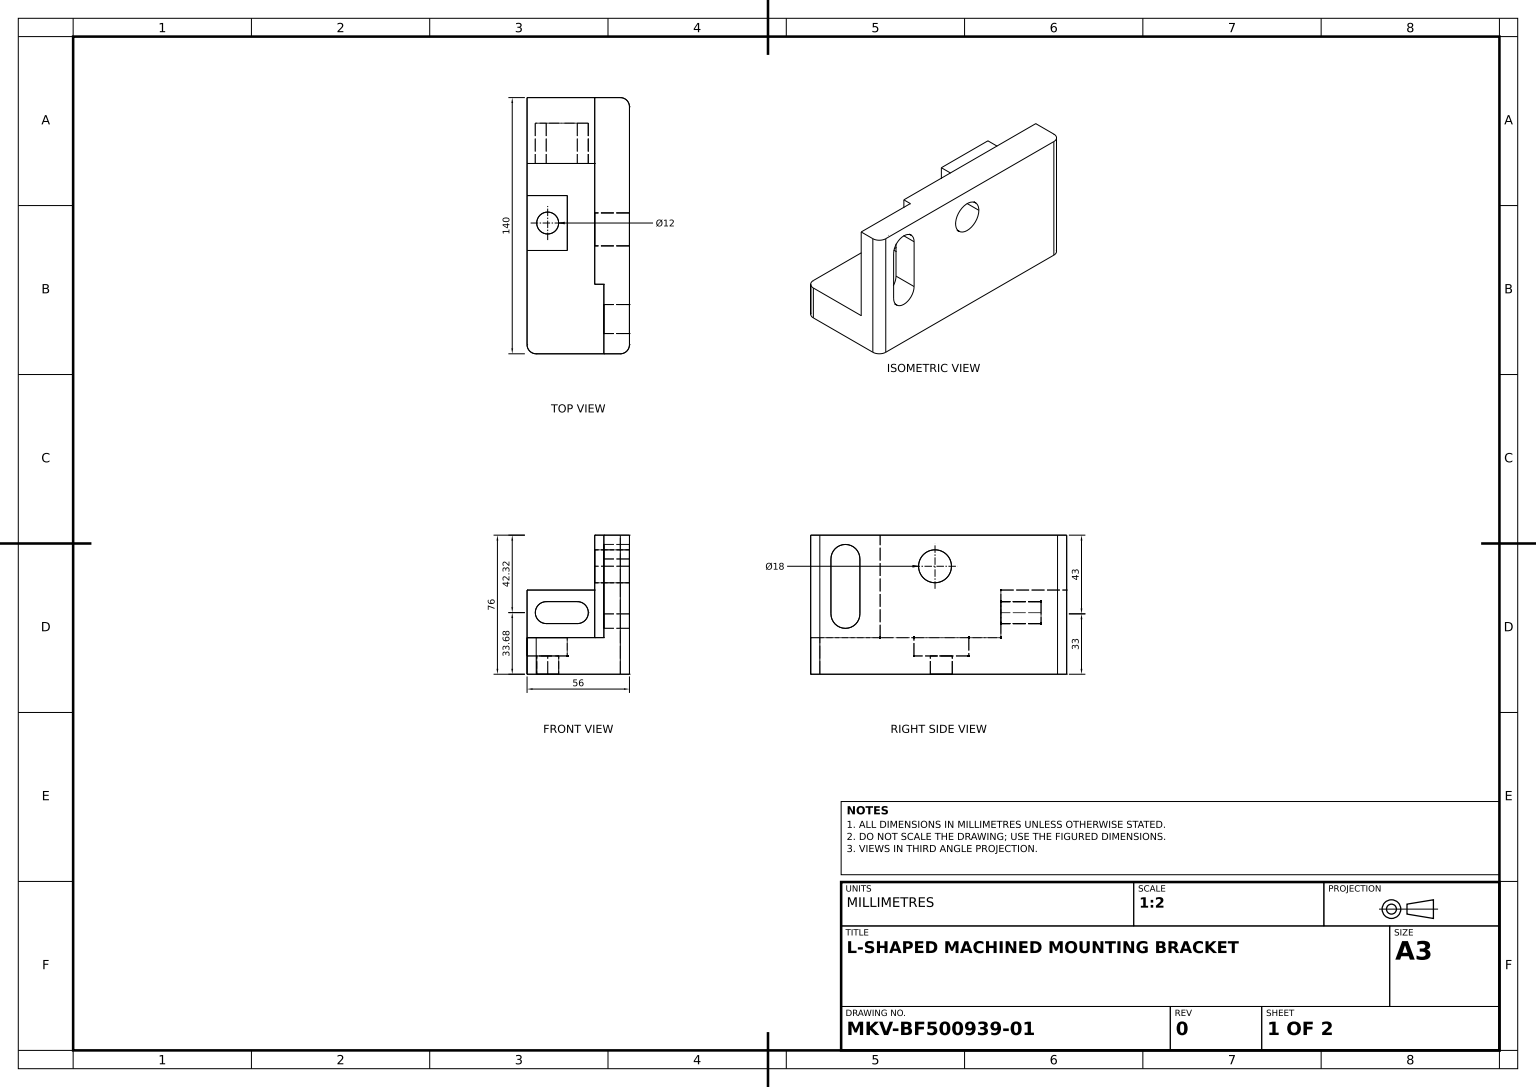
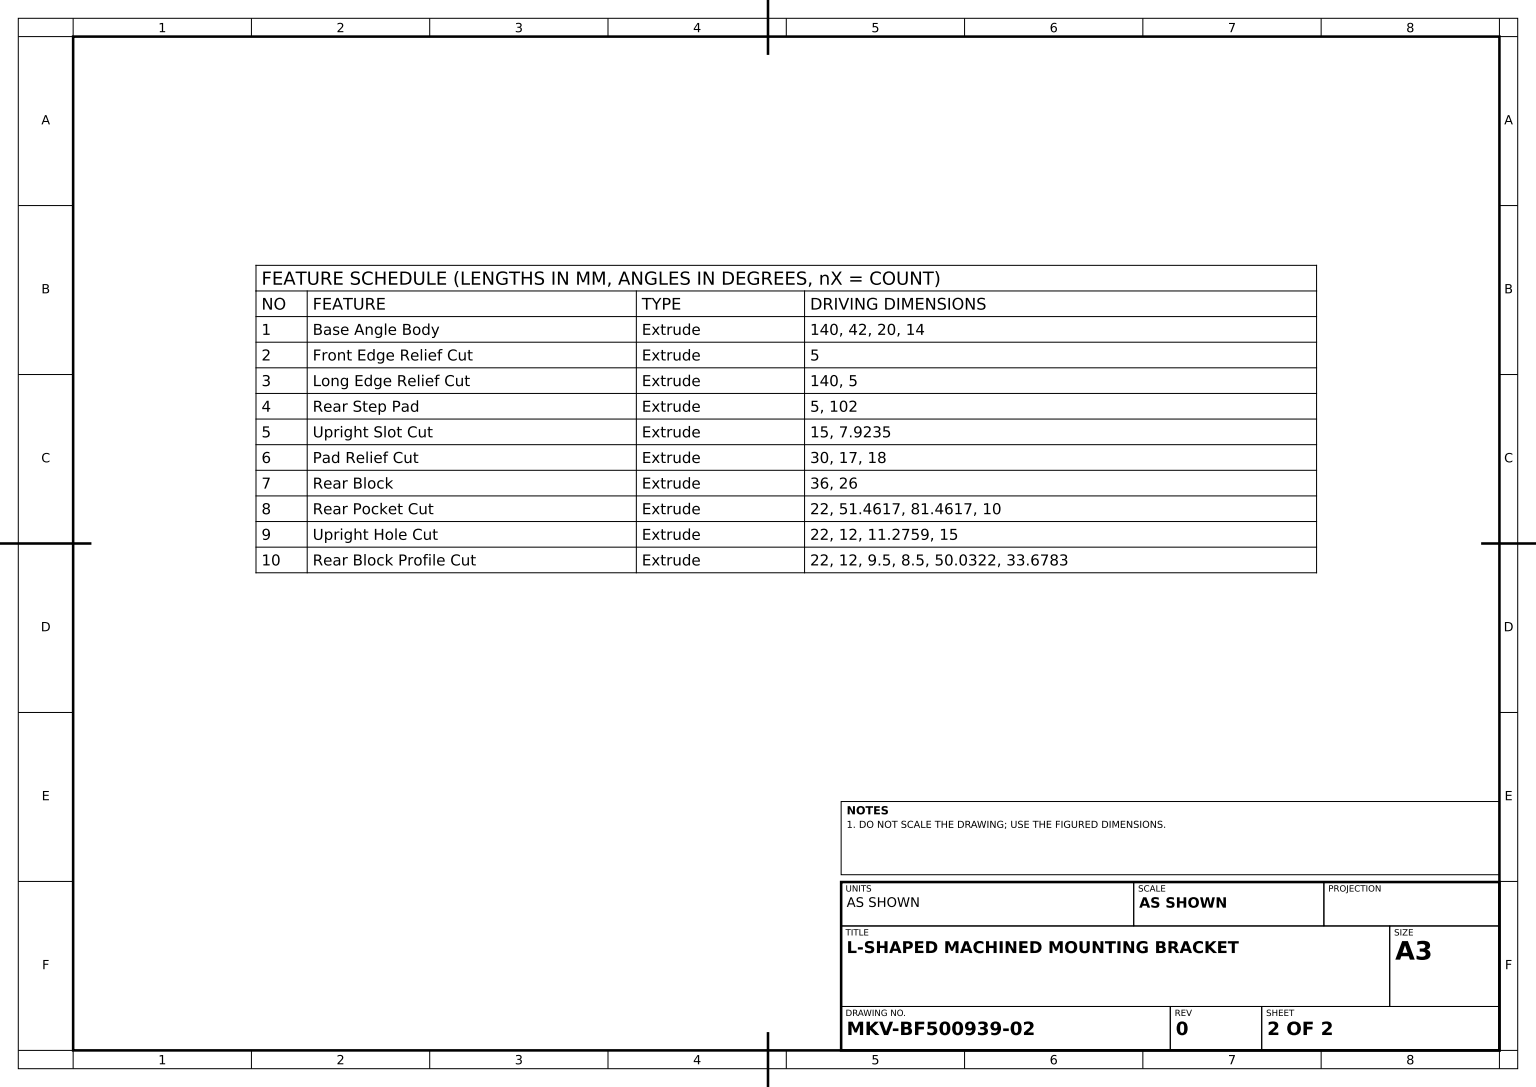
SolidWorks part; units mm, degrees
material "Plain Carbon Steel"
ref_plane "Front Plane" through (0, 0, 0) normal (0, 0, 1) x (1, 0, 0)
ref_plane "Top Plane" through (0, 0, 0) normal (0, 1, 0) x (1, 0, 0)
ref_plane "Right Plane" through (0, 0, 0) normal (1, 0, 0) x (0, 0, -1)
sketch "Base Angle Profile Sketch" plane through (0, 0, 0) normal (0, 0, 1) x (1, 0, 0)
  line L0 (0, 0) -> (-56, 0)
  line L1 (-56, 0) -> (-56, 20)
  line L2 (-56, 20) -> (-14, 20)
  line L3 (-14, 20) -> (-14, 76)
  line L4 (-14, 76) -> (0, 76)
  line L5 (0, 76) -> (0, 0)
  dimension "D1" = 42
  dimension "D2" = 20
  dimension "D3" = 14
extrude "Base Angle Body" add sketch "Base Angle Profile Sketch" along normal mid plane 140
sketch "Front Edge Relief Sketch" plane through (0, 76, 0) normal (0, 1, 0) x (1, 0, 0)
  line L0 (-5, 70) -> (0, 70)
  line L2 (0, 70) -> (0, 65)
  line L4 (0, 0) -> (-56, 0) construction
  line L5 (-56, -70) -> (-56, 70) construction
  line L6 (0, -70) -> (0, -65)
  line L7 (-5, -70) -> (0, -70)
  arc A0 (0, 65) -> (-5, 70) centre (-5, 65) ccw
  arc A1 (0, -65) -> (-5, -70) centre (-5, -65) cw
  dimension "D1" = 5
extrude "Front Edge Relief Cut" cut sketch "Front Edge Relief Sketch" against normal through all
sketch "Long Edge Relief Sketch" plane through (0, 20, 0) normal (0, 1, 0) x (1, 0, 0)
  line L0 (-56, -65) -> (-56, -70)
  line L2 (-56, -70) -> (-51, -70)
  arc A0 (-56, -65) -> (-51, -70) centre (-51, -65) ccw
  dimension "D1" = 5
extrude "Long Edge Relief Cut" cut sketch "Long Edge Relief Sketch" against normal blind 140
sketch "Rear Step Pad Sketch" plane through (-14, 0, 0) normal (-1, 0, 0) x (0, 0, 1)
  line L2 (70, 76) -> (-70, 76) construction
  line L3 (32, 76) -> (32, 20)
  line L4 (65, 20) -> (-70, 20) construction
  line L6 (32, 76) -> (-70, 76)
  line L7 (-70, 76) -> (-70, 20)
  line L8 (-70, 20) -> (32, 20)
  line L9 (-70, 76) -> (-70, 20) construction
  dimension "D1" = 102
extrude "Rear Step Pad" add sketch "Rear Step Pad Sketch" along normal blind 5
sketch "Upright Slot Sketch" plane through (-14, 0, 0) normal (-1, 0, 0) x (0, 0, 1)
  line L0 (51, 76) -> (51, 20) construction
  line L1 (70, 76) -> (32, 76) construction
  line L2 (70, 20) -> (32, 20) construction
  line L3 (51, 33) -> (51, 63) construction
  line L4 (43.0765, 33) -> (43.0765, 63)
  line L5 (58.9235, 33) -> (58.9235, 63)
  arc A0 (43.0765, 33) -> (58.9235, 33) centre (51, 33) ccw
  arc A1 (58.9235, 63) -> (43.0765, 63) centre (51, 63) ccw
  point P8 (51, 48)
  dimension "D2" = 7.9235
  dimension "D1" = 15
extrude "Upright Slot Cut" cut sketch "Upright Slot Sketch" against normal through all
sketch "Pad Relief Sketch" plane through (-19, 0, 0) normal (-1, 0, 0) x (0, 0, 1)
  line L0 (32, 76) -> (2, 76) construction
  line L1 (32, 76) -> (-70, 76) construction
  line L2 (2, 76) -> (2, 59) construction
  circle A0 centre (2, 59) radius 9
  dimension "D1" = 30
  dimension "D3" = 18
  dimension "D2" = 17
extrude "Pad Relief Cut" cut sketch "Pad Relief Sketch" against normal through all
sketch "Rear Block Sketch" plane through (0, 0, -70) normal (0, 0, -1) x (-1, 0, 0)
  line L0 (56, 20) -> (56, 46)
  line L1 (56, 46) -> (19, 46)
  line L2 (19, 76) -> (19, 20) construction
  line L3 (19, 46) -> (19, 20)
  line L4 (19, 20) -> (56, 20)
  line L5 (19, 20) -> (56, 20) construction
  dimension "D1" = 26
extrude "Rear Block" add sketch "Rear Block Sketch" against normal blind 36
sketch "Rear Pocket Sketch" plane through (-56, 0, 0) normal (-1, 0, 0) x (0, 0, 1)
  line L0 (65, 20) -> (-34, 20) construction
  line L1 (-34, 20) -> (32, 20) construction
  line L2 (-16.4617, 20) -> (-16.4617, 10)
  line L3 (-16.4617, 10) -> (13.5383, 10)
  line L4 (13.5383, 10) -> (13.5383, 20)
  line L5 (-16.4617, 20) -> (13.5383, 20)
  dimension "D1" = 51.4617
  dimension "D2" = 81.4617
  dimension "D3" = 10
extrude "Rear Pocket Cut" cut sketch "Rear Pocket Sketch" against normal blind 22
sketch "Upright Hole Sketch" plane through (0, 10, 0) normal (0, 1, 0) x (1, 0, 0)
  line L0 (-56, 16.4617) -> (-56, -13.5383) construction
  circle A0 centre (-44.7241, 1.4617) radius 6
  dimension "D1" = 12
  dimension "D2" = 11.2759
  dimension "D3" = 15
extrude "Upright Hole Cut" cut sketch "Upright Hole Sketch" against normal blind 22
sketch "Rear Block Profile Sketch" plane through (0, 0, -34) normal (0, 0, 1) x (1, 0, 0)
  line L0 (-28.5, 33.6783) -> (-37, 33.6783) construction
  line L2 (-19, 20) -> (-19, 76) construction
  line L3 (-19, 33.6783) -> (-28.5, 33.6783) construction
  line L4 (-45.5, 33.6783) -> (-28.5, 33.6783) construction
  line L5 (-45.5, 39.6783) -> (-28.5, 39.6783)
  line L6 (-45.5, 27.6783) -> (-28.5, 27.6783)
  arc A0 (-45.5, 39.6783) -> (-45.5, 27.6783) centre (-45.5, 33.6783) ccw
  arc A1 (-28.5, 27.6783) -> (-28.5, 39.6783) centre (-28.5, 33.6783) ccw
  point P3 (-37, 33.6783)
  dimension "D2" = 9.5
  dimension "D1" = 12
  dimension "D3" = 8.5
  dimension "D4" = 50.0322
  dimension "D5" = 33.6783
extrude "Rear Block Profile Cut" cut sketch "Rear Block Profile Sketch" against normal blind 22
